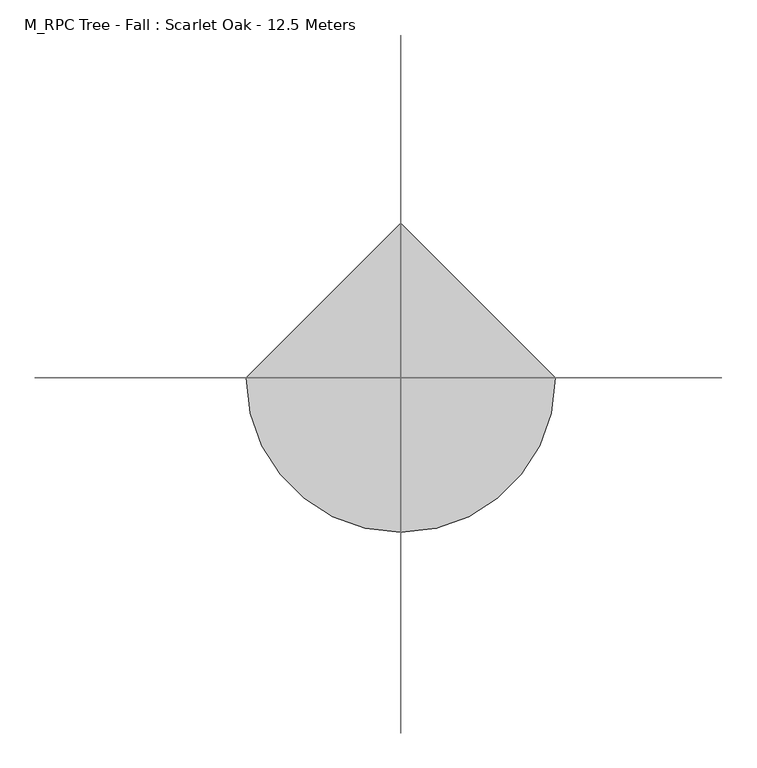
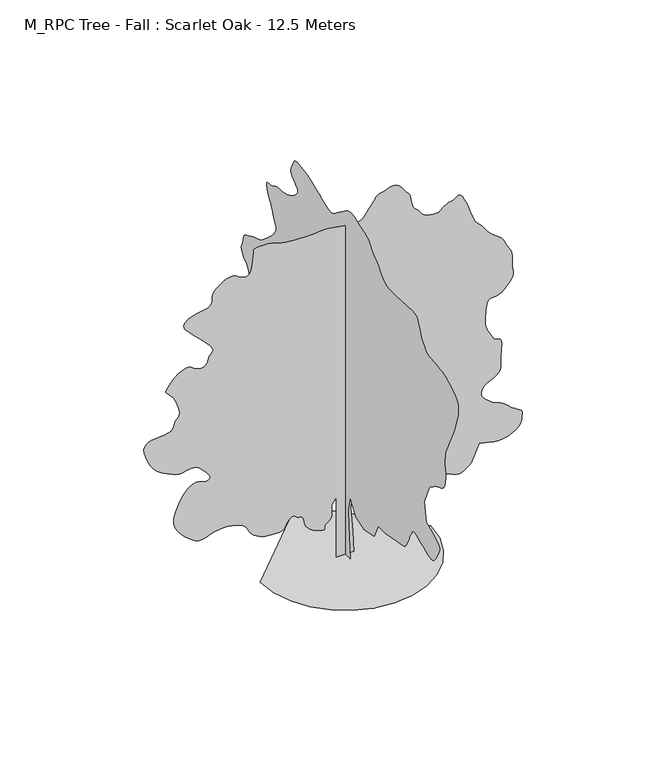
"""IFC4 building model written with IfcOpenShell, lengths in millimetres: geographic element geometry, M_RPC Tree - Fall : Scarlet Oak - 12.5 Meters."""

from ifc_helpers import new_model, si_unit, origin, place, context, project, spatial, triangles, source, transform, mapped, element, save


def m_rpc_tree_fall_scarlet_oak_12_5_meters_78a4568a(model_context):
    return source(origin(), model_context, "Body", "Tessellation", [
        triangles([(0.0172504, 306.0074844, 0.0), (0.0172504, -293.5650026, 0.0), (0.0172504, -196.8600042, 1141.1200275), (0.0172504, -177.5185068, 1682.6674953), (0.0172504, -293.5650026, 2185.5350567), (0.0172504, -603.0224945, 1682.6674953), (0.0172504, -1105.8875124, 1527.9400211), (0.0172504, -1686.1174301, 1663.3275421), (0.0172504, -1918.2099495, 2146.8525341), (0.0172504, -2324.3725124, 2146.8525341), (0.0172504, -3446.150116, 2359.6049549), (0.0172504, -3487.4249222, 2409.394939), (0.0172504, -3527.7000801, 2459.5225479), (0.0172504, -3565.9250725, 2510.3249702), (0.0172504, -3601.0999603, 2562.1500046), (0.0172504, -3632.2250954, 2615.3249565), (0.0172504, -3658.2749588, 2670.2000954), (0.0172504, -3678.2499023, 2727.0751122), (0.0172504, -3697.649881, 2785.6750237), (0.0172504, -3722.1251312, 2845.2748741), (0.0172504, -3750.8251236, 2905.7249634), (0.0172504, -3782.89991, 2966.8500114), (0.0172504, -3817.5251221, 3028.475029), (0.0172504, -3853.8249413, 3090.4500252), (0.0172504, -3890.9999977, 3152.5750122), (0.0172504, -3908.7000801, 3172.6499496), (0.0172504, -3933.1750397, 3188.8501236), (0.0172504, -3971.1750458, 3197.2499016), (0.0172504, -4029.4749756, 3193.9751015), (0.0172504, -4114.8499969, 3175.1500877), (0.0172504, -4234.0499886, 3136.8500999), (0.0172504, -4393.8501183, 3075.2250824), (0.0172504, -4562.5749939, 3002.6998581), (0.0172504, -4706.2499451, 2937.9750298), (0.0172504, -4828.2750549, 2886.4249786), (0.0172504, -4932.0251175, 2853.4999535), (0.0172504, -5020.8999252, 2844.5999153), (0.0172504, -5098.249855, 2865.125116), (0.0172504, -5167.5002792, 2920.4999336), (0.0172504, -5237.3750839, 3007.7251328), (0.0172504, -5309.5997452, 3113.9000473), (0.0172504, -5377.1002762, 3229.5499649), (0.0172504, -5432.7497864, 3345.1998825), (0.0172504, -5469.4498718, 3451.3750877), (0.0172504, -5480.1248016, 3538.6249947), (0.0172504, -5457.6250122, 3597.424894), (0.0172504, -5402.6498795, 3641.7000984), (0.0172504, -5323.3000717, 3691.0249947), (0.0172504, -5223.6747574, 3744.5999222), (0.0172504, -5107.774855, 3801.5499344), (0.0172504, -4979.7251129, 3861.0500816), (0.0172504, -4843.5499947, 3922.2251266), (0.0172504, -4703.3251236, 3984.2501198), (0.0172504, -4587.2749397, 4641.8500969), (0.0172504, -4877.3749649, 5318.7747665), (0.0172504, -4886.5249878, 5331.7001404), (0.0172504, -4900.7252838, 5347.4747589), (0.0172504, -4925.0999588, 5369.0251877), (0.0172504, -4964.6748688, 5399.20009), (0.0172504, -5024.5502838, 5440.8498734), (0.0172504, -5109.8247299, 5496.8999405), (0.0172504, -5225.5252258, 5570.225116), (0.0172504, -5351.0501221, 5636.6501312), (0.0172504, -5462.3497238, 5680.0498077), (0.0172504, -5559.4501923, 5715.3499786), (0.0172504, -5642.3497833, 5757.424736), (0.0172504, -5711.0252426, 5821.1499161), (0.0172504, -5765.4998245, 5921.4001923), (0.0172504, -5805.7502747, 6073.0752365), (0.0172504, -5829.0500153, 6222.0498642), (0.0172504, -5835.7501877, 6317.5748474), (0.0172504, -5830.6249191, 6379.6001312), (0.0172504, -5818.3750854, 6428.1000778), (0.0172504, -5803.7748138, 6483.0252136), (0.0172504, -5791.5499786, 6564.3249023), (0.0172504, -5786.4247101, 6692.0002487), (0.0172504, -5788.2251816, 6832.849791), (0.0172504, -5796.1252808, 6949.6752182), (0.0172504, -5813.8247818, 7056.3751007), (0.0172504, -5845.0502014, 7166.7747574), (0.0172504, -5893.550148, 7294.7750839), (0.0172504, -5963.0249771, 7454.2502335), (0.0172504, -6057.1750443, 7659.049942), (0.0172504, -6146.5748199, 7844.1752701), (0.0172504, -6206.1752518, 7955.8748474), (0.0172504, -6246.4751175, 8024.9502823), (0.0172504, -6277.9999374, 8082.1752777), (0.0172504, -6311.225235, 8158.3502792), (0.0172504, -6356.599791, 8284.2751511), (0.0172504, -6424.6752869, 8490.6997604), (0.0172504, -6498.0248795, 8729.4997192), (0.0172504, -6547.3747742, 8935.1499573), (0.0172504, -6565.2498459, 9112.3751862), (0.0172504, -6544.199968, 9265.925116), (0.0172504, -6476.8250107, 9400.5250397), (0.0172504, -6355.6498489, 9520.9002502), (0.0172504, -6173.2249374, 9631.8248749), (0.0172504, -5996.2252762, 9723.0001236), (0.0172504, -5879.7998245, 9785.7747803), (0.0172504, -5799.2250916, 9827.2001587), (0.0172504, -5729.8002594, 9854.4496582), (0.0172504, -5646.85009, 9874.575174), (0.0172504, -5525.6749283, 9894.699527), (0.0172504, -5341.575119, 9921.9501892), (0.0172504, -5144.0999634, 9943.4244598), (0.0172504, -4990.9500092, 9951.725116), (0.0172504, -4869.5998581, 9962.0244873), (0.0172504, -4767.5499825, 9989.5995483), (0.0172504, -4672.2499855, 10049.6505341), (0.0172504, -4571.2000488, 10157.425351), (0.0172504, -4451.8750648, 10328.0998169), (0.0172504, -4347.6750298, 10515.7499908), (0.0172504, -4286.1000092, 10666.5500885), (0.0172504, -4245.8501404, 10783.8254883), (0.0172504, -4205.5749825, 10871.0003998), (0.0172504, -4143.9999619, 10931.4501984), (0.0172504, -4039.7999268, 10968.5502594), (0.0172504, -3871.650016, 10985.7003754), (0.0172504, -2943.2749969, 10927.6748474), (0.0172504, -2772.1499771, 10930.6746643), (0.0172504, -2632.8250511, 10930.2746887), (0.0172504, -2514.4500092, 10937.3254211), (0.0172504, -2406.244986, 10962.6250397), (0.0172504, -2297.3600624, 11017.0496246), (0.0172504, -2176.9724979, 11111.3752625), (0.0172504, -2034.2550465, 11256.4745453), (0.0172504, -1896.7275398, 11403.0249023), (0.0172504, -1793.7050491, 11502.8746216), (0.0172504, -1717.0749882, 11568.5752625), (0.0172504, -1658.7125622, 11612.6248993), (0.0172504, -1610.5025688, 11647.5250946), (0.0172504, -1564.320068, 11685.7995026), (0.0172504, -1512.0500027, 11739.9996826), (0.0172504, -1461.8649845, 11804.0004272), (0.0172504, -1420.8125484, 11863.6002777), (0.0172504, -1379.087479, 11919.1503754), (0.0172504, -1326.8724976, 11970.9495392), (0.0172504, -1254.3574471, 12019.4000702), (0.0172504, -1151.7299904, 12064.7996246), (0.0172504, -1009.182514, 12107.4749268), (0.0172504, -849.1549999, 12154.4999634), (0.0172504, -699.9524792, 12206.6002716), (0.0172504, -560.5600064, 12254.6496643), (0.0172504, -429.9675053, 12289.4998627), (0.0172504, -307.1550161, 12302.0246796), (0.0172504, -191.1079934, 12283.0746735), (0.0172504, -80.8134993, 12223.5248199), (0.0172504, 499.4175176, 11798.0252106), (0.0172504, 562.2325061, 11740.8496307), (0.0172504, 623.0199657, 11688.7504852), (0.0172504, 689.217524, 11646.7751404), (0.0172504, 768.2749804, 11620.0500275), (0.0172504, 867.630035, 11613.6248383), (0.0172504, 994.7275097, 11632.5748444), (0.0172504, 1157.0125168, 11681.9753174), (0.0172504, 1341.1749676, 11755.3254913), (0.0172504, 1526.6899521, 11837.8251068), (0.0172504, 1710.1749733, 11922.0246185), (0.0172504, 1888.2475342, 12000.4500641), (0.0172504, 2057.5249924, 12065.6995697), (0.0172504, 2214.6200546, 12110.3003357), (0.0172504, 2356.1550201, 12126.8249084), (0.0172504, 2484.8875694, 12135.849939), (0.0172504, 2604.4750374, 12156.3754303), (0.0172504, 2712.9251038, 12178.575238), (0.0172504, 2808.1501053, 12192.6755402), (0.0172504, 2888.1748718, 12188.8501923), (0.0172504, 2950.9251114, 12157.2753754), (0.0172504, 2994.400074, 12088.1249451), (0.0172504, 3033.2500282, 12001.2500153), (0.0172504, 3077.8499222, 11921.1246735), (0.0172504, 3119.7499809, 11845.0502472), (0.0172504, 3150.5001389, 11770.3245758), (0.0172504, 3161.6000427, 11694.2745667), (0.0172504, 3144.6249161, 11614.1503876), (0.0172504, 3091.124984, 11527.2498779), (0.0172504, 3009.2500397, 11447.6245056), (0.0172504, 2921.5998665, 11385.2504059), (0.0172504, 2841.4251091, 11331.3502075), (0.0172504, 2781.8749649, 11277.1000305), (0.0172504, 2756.1750801, 11213.7248291), (0.0172504, 2777.4749428, 11132.4251404), (0.0172504, 2859.0249069, 11024.3747589), (0.0172504, 2971.6250107, 10916.7255157), (0.0172504, 3077.7999252, 10838.2000763), (0.0172504, 3178.2249001, 10782.3), (0.0172504, 3273.574894, 10742.6745117), (0.0172504, 3364.5248657, 10712.8251709), (0.0172504, 3451.7750633, 10686.4000397), (0.0172504, 3535.9498672, 10656.8995148), (0.0172504, 3620.024968, 10634.1753204), (0.0172504, 3706.4749237, 10626.6746155), (0.0172504, 3795.2750267, 10625.9502411), (0.0172504, 3886.4499847, 10623.5248077), (0.0172504, 3980.0000885, 10610.9499939), (0.0172504, 4075.9250473, 10579.7495728), (0.0172504, 4174.1998627, 10521.5252197), (0.0172504, 4275.775058, 10469.80047), (0.0172504, 4375.6250679, 10451.2504395), (0.0172504, 4465.0001358, 10446.8995422), (0.0172504, 4535.0999268, 10437.8245148), (0.0172504, 4577.0999794, 10405.075351), (0.0172504, 4582.2249573, 10329.6753021), (0.0172504, 4541.7001053, 10192.7255219), (0.0172504, 4481.7999825, 10048.5994354), (0.0172504, 4432.0751106, 9951.4995483), (0.0172504, 4388.424868, 9882.1247131), (0.0172504, 4346.8250816, 9821.224942), (0.0172504, 4303.1751297, 9749.5002502), (0.0172504, 4253.4249687, 9647.6750702), (0.0172504, 4193.550135, 9496.4499985), (0.0172504, 4130.2749275, 9347.6997757), (0.0172504, 4075.8250534, 9253.7502777), (0.0172504, 4034.1999779, 9195.999733), (0.0172504, 4009.500032, 9155.8498581), (0.0172504, 4005.7749687, 9114.7000443), (0.0172504, 4027.1001205, 9053.900267), (0.0172504, 4077.4999512, 8954.8999146), (0.0172504, 4167.2249977, 8823.6747849), (0.0172504, 4293.1248711, 8684.3501495), (0.0172504, 4439.3499573, 8545.349913), (0.0172504, 4589.9500671, 8415.1497208), (0.0172504, 4729.0750053, 8302.2002197), (0.0172504, 4840.7748734, 8214.9747299), (0.0172504, 4909.1747681, 8161.9000626), (0.0172504, 4969.9001312, 8128.6997635), (0.0172504, 5061.0747986, 8095.1500671), (0.0172504, 5170.5250946, 8060.9248306), (0.0172504, 5286.0750183, 8025.675238), (0.0172504, 5395.524733, 7989.0751465), (0.0172504, 5486.6999817, 7950.8001572), (0.0172504, 5547.4247635, 7910.4747116), (0.0172504, 5598.275148, 7876.9750122), (0.0172504, 5663.0252655, 7853.2997131), (0.0172504, 5734.1749924, 7830.2999542), (0.0172504, 5804.3247803, 7798.8251312), (0.0172504, 5866.0250839, 7749.7752182), (0.0172504, 5911.8001968, 7673.9751938), (0.0172504, 5934.2499893, 7562.325032), (0.0172504, 5952.6250305, 7450.1749008), (0.0172504, 5984.1998474, 7370.8500916), (0.0172504, 6018.4750809, 7312.1501862), (0.0172504, 6045.000206, 7261.899765), (0.0172504, 6053.2252853, 7207.9501511), (0.0172504, 6032.699794, 7138.074765), (0.0172504, 5972.9249542, 7040.1249298), (0.0172504, 5898.7248322, 6948.3747162), (0.0172504, 5838.7250061, 6893.5251572), (0.0172504, 5788.2001831, 6857.9500031), (0.0172504, 5742.4000717, 6824.0497467), (0.0172504, 5696.6249588, 6774.2498795), (0.0172504, 5646.1001358, 6690.9747299), (0.0172504, 5586.0997284, 6556.5997925), (0.0172504, 5520.7002319, 6421.9998688), (0.0172504, 5460.6998245, 6337.1498154), (0.0172504, 5411.5249191, 6283.075209), (0.0172504, 5378.6001846, 6240.824881), (0.0172504, 5367.3247101, 6191.4999847), (0.0172504, 5383.09991, 6116.0999359), (0.0172504, 5431.3748703, 5995.7247253), (0.0172504, 5495.5000259, 5864.0502045), (0.0172504, 5555.8748291, 5761.8250488), (0.0172504, 5613.5747955, 5680.5747757), (0.0172504, 5669.5498672, 5611.8249023), (0.0172504, 5724.8749786, 5547.1497803), (0.0172504, 5780.5250702, 5478.0749268), (0.0172504, 5837.5250793, 5396.1502762), (0.0172504, 5903.6751114, 5315.3499756), (0.0172504, 5980.6500641, 5249.4249298), (0.0172504, 6060.324852, 5189.6000931), (0.0172504, 6134.5999695, 5127.0498413), (0.0172504, 6195.3247513, 5053.0252899), (0.0172504, 6234.4002731, 4958.675235), (0.0172504, 6243.7002869, 4835.2499199), (0.0172504, 6251.5248093, 4738.3250221), (0.0172504, 6280.349794, 4706.349939), (0.0172504, 6313.2251129, 4704.825032), (0.0172504, 6333.2500534, 4699.2500816), (0.0172504, 6323.4750687, 4655.0998695), (0.0172504, 6267.0500244, 4537.8750481), (0.0172504, 6146.999794, 4313.0501083), (0.0172504, 6021.4748978, 4060.8750938), (0.0172504, 5945.6998718, 3875.3750793), (0.0172504, 5898.3248566, 3742.6250427), (0.0172504, 5858.0749878, 3648.7999557), (0.0172504, 5803.5998245, 3580.0000854), (0.0172504, 5713.6000854, 3522.3751144), (0.0172504, 5566.7747452, 3462.0500175), (0.0172504, 5397.250209, 3413.1000984), (0.0172504, 5248.0500137, 3392.5748978), (0.0172504, 5111.025238, 3390.9999939), (0.0172504, 4978.0752136, 3398.9000931), (0.0172504, 4841.0498566, 3406.7749031), (0.0172504, 4691.8499519, 3405.1999992), (0.0172504, 4522.3501236, 3384.6750893), (0.0172504, 4353.2999771, 3366.3000481), (0.0172504, 4207.2498802, 3370.2500977), (0.0172504, 4078.7998718, 3385.7000267), (0.0172504, 3962.5249924, 3401.8249146), (0.0172504, 3853.0249901, 3407.8001312), (0.0172504, 3744.8749054, 3392.799884), (0.0172504, 3632.6500694, 3346.0001244), (0.0172504, 3525.249939, 3296.2499634), (0.0172504, 3436.4251282, 3270.2000999), (0.0172504, 3368.249929, 3253.6249489), (0.0172504, 3322.75009, 3232.3250862), (0.0172504, 3301.9499062, 3192.0499283), (0.0172504, 3307.8751259, 3118.6500481), (0.0172504, 3342.5500443, 2997.8498634), (0.0172504, 3398.475119, 2869.5251381), (0.0172504, 3465.5750931, 2778.7248665), (0.0172504, 3542.0000793, 2719.2500084), (0.0172504, 3625.8499031, 2684.8000763), (0.0172504, 3715.274968, 2669.1248703), (0.0172504, 3808.4250961, 2665.9500641), (0.0172504, 3903.4251114, 2669.0498749), (0.0172504, 4270.9250633, 2262.8999565), (0.0172504, 4299.7250496, 2217.1674282), (0.0172504, 4327.3501076, 2170.5925095), (0.0172504, 4352.6250183, 2122.3249615), (0.0172504, 4374.3248566, 2071.5174522), (0.0172504, 4391.2999832, 2017.3300621), (0.0172504, 4402.3498901, 1958.9125523), (0.0172504, 4406.2999397, 1895.4200615), (0.0172504, 4405.6249809, 1829.2200325), (0.0172504, 4400.8999786, 1763.6974331), (0.0172504, 4388.0248924, 1699.5299835), (0.0172504, 4362.9999664, 1637.3900265), (0.0172504, 4321.7248695, 1577.9574623), (0.0172504, 4260.1501396, 1521.9075405), (0.0172504, 4174.1998627, 1469.9175453), (0.0172504, 4092.2249245, 1425.7650078), (0.0172504, 4034.5999535, 1391.4249527), (0.0172504, 3985.4250481, 1364.8675621), (0.0172504, 3928.800016, 1344.0599659), (0.0172504, 3848.8499542, 1326.9749622), (0.0172504, 3729.6499626, 1311.5799717), (0.0172504, 3555.3001396, 1295.8475018), (0.0172504, 3356.9750359, 1298.1024513), (0.0172504, 3174.2251442, 1332.8375404), (0.0172504, 3003.6500908, 1392.27243), (0.0172504, 2841.8750816, 1468.6199501), (0.0172504, 2685.525032, 1554.1049938), (0.0172504, 2531.1748604, 1640.9425713), (0.0172504, 2375.4949734, 1721.3500179), (0.0172504, 2236.6675461, 1794.4849434), (0.0172504, 2129.3050587, 1863.5599422), (0.0172504, 2044.6099377, 1926.8850014), (0.0172504, 1973.7875164, 1982.7650208), (0.0172504, 1908.0399307, 2029.5099873), (0.0172504, 1838.5700432, 2065.4300331), (0.0172504, 1756.5824604, 2088.8300583), (0.0172504, 1666.4174698, 2108.5650455), (0.0172504, 1577.6074837, 2133.0375343), (0.0172504, 1489.134977, 2159.8799366), (0.0172504, 1399.9875114, 2186.7200134), (0.0172504, 1309.1449459, 2211.1925022), (0.0172504, 1215.5975309, 2230.9274895), (0.0172504, 1118.3299942, 2243.5575325), (0.0172504, 1018.8625191, 2250.1549496), (0.0172504, 919.3925005, 2253.7074944), (0.0172504, 819.9250254, 2254.7225487), (0.0172504, 720.4574776, 2253.7074944), (0.0172504, 620.9900024, 2251.1700039), (0.0172504, 521.5199839, 2247.6174591), (0.0172504, 422.0525087, 2243.5575325), (0.0172504, 228.6430025, 1953.4425373), (0.0172504, 189.960498, 1508.6000679), (280.4450004, 0.0006008, 0.0092122), (-299.7850081, 0.0006008, 0.0092122), (-299.7850081, 0.0004756, 2127.5199932), (-454.5149895, 0.0004756, 1914.7700432), (-454.5149895, 0.0005007, 1682.6775238), (-450.9625174, 0.0005007, 1628.8274677), (-450.9625174, 0.0005007, 1575.1449886), (-458.0674979, 0.0005007, 1521.8024597), (-475.8274967, 0.0005257, 1468.967458), (-507.8000001, 0.0005257, 1416.8100311), (-557.5350094, 0.0005257, 1365.4949947), (-628.5824896, 0.0005257, 1315.1974834), (-684.2375227, 0.0005257, 1262.982502), (-699.6325132, 0.0005257, 1210.0900183), (-696.0799685, 0.0005257, 1162.9524885), (-694.8950117, 0.0005257, 1127.990015), (-717.3950191, 0.0005257, 1111.6375248), (-784.8900272, 0.0005257, 1120.3225325), (-918.6974848, 0.0005257, 1160.4700092), (-1071.3399845, 0.0005257, 1223.0050003), (-1185.4125275, 0.0005257, 1293.6575191), (-1267.3425556, 0.0005257, 1371.0799736), (-1323.5625252, 0.0005257, 1453.9125629), (-1360.49748, 0.0005007, 1540.8049335), (-1384.5749348, 0.0005007, 1630.4049877), (-1402.2250202, 0.0005007, 1721.3600464), (-1406.7350647, 0.0005007, 1746.1124599), (-1413.4449749, 0.0005007, 1770.19006), (-1424.5524364, 0.0005007, 1792.9174519), (-1442.2599312, 0.0005007, 1813.6099388), (-1468.7600578, 0.0005007, 1831.5975037), (-1506.2599491, 0.0005007, 1846.2025715), (-1556.9524944, 0.0005007, 1856.7475674), (-1607.6450397, 0.0005007, 1874.1124958), (-1647.5100483, 0.0005007, 1903.3224861), (-1682.3025467, 0.0004756, 1934.9000645), (-1717.7700039, 0.0004756, 1959.3725533), (-1759.6674465, 0.0004756, 1967.2675655), (-1813.7424889, 0.0004756, 1949.1099529), (-1885.7500122, 0.0005007, 1895.4274738), (-1949.0724552, 0.0005007, 1820.3199944), (-1984.9925011, 0.0005007, 1746.902528), (-2011.1000645, 0.0005007, 1679.2374722), (-2044.9875309, 0.0005007, 1621.382428), (-2104.2525181, 0.0005007, 1577.4025543), (-2206.4824699, 0.0005007, 1551.3499294), (-2369.2750042, 0.0005007, 1547.2900028), (-2549.149926, 0.0005007, 1559.2449417), (-2695.2000229, 0.0005007, 1578.979929), (-2813.8250496, 0.0005007, 1607.1750103), (-2911.4999016, 0.0005007, 1644.5025284), (-2994.6250603, 0.0005007, 1691.6425289), (-3069.600135, 0.0005007, 1749.2724415), (-3142.9250198, 0.0005007, 1818.0650448), (-3205.1000038, 0.0005007, 1893.5100037), (-3249.7248962, 0.0004756, 1969.2975288), (-3287.549913, 0.0004756, 2043.389954), (-3329.4499718, 0.0004756, 2113.7625481), (-3386.2249947, 0.0004756, 2178.3824409), (-3468.7249008, 0.0004756, 2235.2224308), (-3587.7499031, 0.0004756, 2282.2499382), (-3707.4248657, 0.0004756, 2317.9974655), (-3794.2500893, 0.0004506, 2343.2600224), (-3862.8249733, 0.0004506, 2359.3875263), (-3927.6750847, 0.0004506, 2367.7325111), (-4003.3251183, 0.0004506, 2369.6499813), (-4104.3750549, 0.0004506, 2366.4924706), (-4245.3498802, 0.0004506, 2359.6125126), (-4400.3500122, 0.0004506, 2335.1974331), (-4538.1250328, 0.0004756, 2289.8050003), (-4665.0501343, 0.0004756, 2240.3524956), (-4787.5749229, 0.0004756, 2203.7574909), (-4912.1501678, 0.0004756, 2196.9349422), (-5045.1501892, 0.0004756, 2236.7999508), (-5193.0498825, 0.0004506, 2340.2725594), (-5347.7997391, 0.0004506, 2478.6475433), (-5490.6747391, 0.0004506, 2615.9999153), (-5612.2498764, 0.0004256, 2758.4499413), (-5703.0251495, 0.0004256, 2912.049868), (-5753.5499725, 0.0004256, 3082.8999046), (-5754.3499237, 0.0004005, 3277.0999695), (-5695.9250015, 0.0004005, 3500.7249825), (-5598.1501556, 0.0003755, 3726.2748779), (-5489.1998291, 0.0003755, 3919.6999901), (-5372.1499969, 0.0003505, 4077.2499664), (-5250.0248932, 0.0003505, 4195.2000343), (-5125.8499146, 0.0003505, 4269.8501289), (-5002.6998734, 0.0003505, 4297.4998947), (-4883.6001663, 0.0003505, 4274.3751434), (-4771.2750458, 0.0003505, 4235.4749016), (-4671.8250114, 0.0003505, 4218.8750427), (-4593.3248611, 0.0003505, 4225.6499199), (-4543.9249695, 0.0003505, 4256.7750549), (-4531.7501312, 0.0003505, 4313.2750946), (-4564.9001427, 0.0003505, 4396.1749763), (-4651.5000893, 0.0003254, 4506.4749298), (-4752.500029, 0.0003254, 4617.0998634), (-4829.4749817, 0.0003254, 4702.3498924), (-4891.5502625, 0.0003254, 4765.2751213), (-4947.8747314, 0.0003254, 4808.9250732), (-5007.6001556, 0.0003254, 4836.325145), (-5079.8248169, 0.0003004, 4850.5498581), (-5173.7248993, 0.0003004, 4854.5999016), (-5270.0248352, 0.0003254, 4845.5248741), (-5349.7751999, 0.0003254, 4824.5999886), (-5422.3998367, 0.0003254, 4801.3249557), (-5497.39991, 0.0003254, 4785.1250725), (-5584.2248428, 0.0003254, 4785.5250481), (-5692.3752182, 0.0003254, 4811.9748871), (-5831.3248764, 0.0003004, 4873.9498833), (-5978.7751785, 0.0003004, 4948.0997177), (-6108.6248108, 0.0003004, 5012.4248611), (-6224.6252884, 0.0003004, 5078.4748993), (-6330.4502243, 0.0003004, 5157.6997147), (-6429.8749695, 0.0003004, 5261.5997681), (-6526.574881, 0.0002754, 5401.7249359), (-6624.2997299, 0.0002754, 5589.5750977), (-6705.1000305, 0.0002503, 5784.4998276), (-6749.7002151, 0.0002503, 5941.2001465), (-6759.8001801, 0.0002503, 6064.0752045), (-6737.074823, 0.0002253, 6157.4997345), (-6683.2252029, 0.0002253, 6225.9002106), (-6599.9500534, 0.0002253, 6273.6502029), (-6488.899855, 0.0002253, 6305.1750229), (-6357.7997177, 0.0002253, 6323.2750809), (-6219.2750336, 0.0002253, 6333.9500107), (-6082.4002487, 0.0002253, 6346.2748398), (-5956.3748016, 0.0002253, 6369.4501694), (-5850.3248795, 0.0002253, 6412.5998611), (-5773.3499268, 0.0002253, 6484.8251038), (-5734.5999664, 0.0002003, 6595.2997559), (-5705.9749695, 0.0002003, 6701.9752213), (-5661.749762, 0.0002003, 6771.4500504), (-5614.8497177, 0.0002003, 6825.7002274), (-5578.0752182, 0.0002003, 6886.6999924), (-5564.3248947, 0.0001752, 6976.4747452), (-5586.4252899, 0.0001752, 7116.9998886), (-5657.2500366, 0.0001752, 7330.2502441), (-5757.5497284, 0.0001502, 7540.3002136), (-5853.4752686, 0.0001502, 7672.5252823), (-5935.8498917, 0.0001502, 7750.975145), (-5995.5747345, 0.0001252, 7799.6250824), (-6023.4747757, 0.0001252, 7842.5247894), (-6010.4499893, 0.0001252, 7903.7251236), (-5947.3497711, 0.0001252, 8007.2002029), (-5845.6501648, 0.0001252, 8136.3248795), (-5728.0247864, 0.0001001, 8253.9502579), (-5602.2749039, 0.0001001, 8353.3000076), (-5476.1750427, 0.0001001, 8427.6251221), (-5357.5497253, 0.0001001, 8470.1248535), (-5254.1252243, 0.0001001, 8474.0751938), (-5173.7248993, 0.0001001, 8432.6998123), (-5094.9000595, 0.0001001, 8371.00009), (-4997.8001724, 0.0001001, 8322.8501221), (-4892.5751999, 0.0001001, 8294.6500992), (-4789.3751038, 0.0001001, 8292.850209), (-4698.375135, 0.0001001, 8323.8750595), (-4629.6999664, 0.0001001, 8394.1248413), (-4593.5001411, 0.0001001, 8510.0497421), (-4560.3251312, 0.0001001, 8620.5749725), (-4508.2251137, 7.51e-05, 8686.1000427), (-4458.4999512, 7.51e-05, 8730.3002518), (-4432.4500877, 7.51e-05, 8776.8747345), (-4451.4000938, 7.51e-05, 8849.4999527), (-4536.6501228, 7.51e-05, 8971.8750412), (-4709.5500343, 5.01e-05, 9167.6497192), (-4926.3498825, 5.01e-05, 9388.800174), (-5120.1502625, 2.5e-05, 9575.0998489), (-5277.4249649, 2.5e-05, 9731.9751572), (-5384.5998184, 2.5e-05, 9864.8246063), (-5428.2000641, 0.0, 9979.0746094), (-5394.6497864, 0.0, 10080.1254181), (-5270.4248108, 0.0, 10173.3755402), (-5104.7500397, 0.0, 10245.2246429), (-4956.3497955, 0.0, 10286.2744629), (-4825.8749107, 0.0, 10308.3754395), (-4714.0000534, -2.5e-05, 10323.3745239), (-4621.3998917, -2.5e-05, 10343.1000641), (-4548.7749641, -2.5e-05, 10379.4245911), (-4496.7749405, -2.5e-05, 10444.1497101), (-4470.8500694, -2.5e-05, 10520.7252686), (-4466.9000198, -2.5e-05, 10587.8246613), (-4471.4000359, -2.5e-05, 10650.1999237), (-4470.8500694, -2.5e-05, 10712.5751862), (-4451.6750771, -5.01e-05, 10779.6745789), (-4400.3500122, -5.01e-05, 10856.2501373), (-4303.3751175, -5.01e-05, 10947.0248291), (-4184.6750954, -5.01e-05, 11036.8495789), (-4076.1250351, -5.01e-05, 11106.7255463), (-3976.0500389, -7.51e-05, 11155.60047), (-3882.7249214, -7.51e-05, 11182.4999908), (-3794.4750755, -7.51e-05, 11186.3997528), (-3709.6000237, -7.51e-05, 11166.2498199), (-3626.4498665, -5.01e-05, 11121.1002502), (-3540.7248665, -5.01e-05, 11065.9001312), (-3452.3250298, -5.01e-05, 11022.8748505), (-3365.6000908, -5.01e-05, 11001.8249725), (-3284.9500717, -5.01e-05, 11012.5998962), (-3214.7999931, -5.01e-05, 11064.9746063), (-3159.5498772, -7.51e-05, 11168.7996643), (-3123.5750381, -7.51e-05, 11333.8500549), (-3102.0998955, -7.51e-05, 11511.0752838), (-3086.6999634, -0.0001001, 11648.0250641), (-3076.3750122, -0.0001001, 11749.4746857), (-3070.125103, -0.0001001, 11820.1250244), (-3066.9000092, -0.0001001, 11864.7246277), (-3065.7250809, -0.0001001, 11888.025531), (-3065.5500916, -0.0001001, 11894.7251221), (-3040.1248993, -0.0001001, 11898.674881), (-2971.0500458, -0.0001001, 11907.3755127), (-2869.1498703, -0.0001001, 11916.0505646), (-2745.2748734, -0.0001001, 11920.0003235), (-2610.2249771, -0.0001001, 11914.4750793), (-2474.8323692, -0.0001001, 11894.7251221), (-2349.935051, -0.0001001, 11856.0495758), (-2235.4100647, -0.0001001, 11813.0254578), (-2120.5474537, -0.0001001, 11781.8494537), (-2000.2725277, -0.0001001, 11760.1251984), (-1869.5075443, -0.0001001, 11745.5249268), (-1723.1824642, -0.0001001, 11735.675528), (-1556.2175102, -0.0001001, 11728.174823), (-1363.5400269, -0.0001001, 11720.6752808), (-1177.5749971, -0.0001001, 11719.599765), (-1024.4249702, -0.0001001, 11728.6747925), (-889.5449764, -0.0001001, 11741.475174), (-758.3875025, -0.0001001, 11751.5745575), (-616.4050352, -0.0001001, 11752.5244995), (-449.0450109, -0.0001001, 11737.9253906), (-241.763259, -0.0001001, 11701.3252991), (-32.2257492, -0.0001001, 11657.8000488), (136.7125037, -0.0001001, 11627.7995544), (271.8174929, -0.0001001, 11613.0248749), (379.8574825, -0.0001001, 11615.1503265), (467.5975121, -0.0001001, 11635.9246399), (541.8025031, -0.0001001, 11676.9744598), (609.2425, -0.0001001, 11739.9996826), (899.3575315, -0.0001252, 12107.4749268), (942.8899761, -0.0001252, 12164.1505371), (977.6249926, -0.0001252, 12217.4496094), (1008.9749685, -0.0001252, 12266.3245331), (1042.3575239, -0.0001252, 12309.7997864), (1083.1825029, -0.0001252, 12346.8498505), (1136.864982, -0.0001252, 12376.4503693), (1208.8150234, -0.0001252, 12397.6002411), (1297.0049892, -0.0001502, 12421.8499237), (1393.3149536, -0.0001502, 12454.2246918), (1494.0224693, -0.0001502, 12483.8752075), (1595.4100307, -0.0001502, 12499.9998047), (1693.7499584, -0.0001502, 12491.7747253), (1785.3225666, -0.0001502, 12448.349469), (1866.410059, -0.0001252, 12358.9246948), (1938.4149662, -0.0001252, 12256.9251068), (2004.3324543, -0.0001252, 12177.5752991), (2062.8075188, -0.0001252, 12112.7746033), (2112.4850098, -0.0001252, 12054.4246765), (2152.0125389, -0.0001252, 11994.3748535), (2180.0375725, -0.0001001, 11924.5000488), (2195.2049606, -0.0001001, 11836.6995941), (2205.7499565, -0.0001001, 11745.7004974), (2220.3550243, -0.0001001, 11669.9248901), (2238.3424438, -0.0001001, 11606.8252533), (2259.0349308, -7.51e-05, 11553.8749969), (2281.7599972, -7.51e-05, 11508.5254395), (2305.8374519, -7.51e-05, 11468.2755707), (2330.5924816, -7.51e-05, 11430.5499664), (2355.6274361, -7.51e-05, 11413.5754211), (2381.680061, -7.51e-05, 11394.2254395), (2409.760033, -7.51e-05, 11370.1501648), (2440.8876389, -7.51e-05, 11338.9753235), (2476.0724098, -7.51e-05, 11298.3254791), (2516.3248947, -7.51e-05, 11245.8251953), (2562.6749725, -7.51e-05, 11179.1246155), (2631.3751396, -5.01e-05, 11115.7249969), (2728.4750267, -5.01e-05, 11072.3253204), (2839.7749191, -5.01e-05, 11045.1246552), (2951.0751022, -5.01e-05, 11030.4755493), (3048.1749893, -5.01e-05, 11024.6003265), (3116.8748657, -5.01e-05, 11023.8247925), (3142.9250198, -5.01e-05, 11024.4003387), (3156.2750771, -5.01e-05, 11038.3250702), (3192.9998703, -5.01e-05, 11074.2252045), (3247.9750031, -5.01e-05, 11123.3501129), (3316.1499115, -7.51e-05, 11176.8503357), (3392.4249069, -7.51e-05, 11225.9752441), (3471.7750053, -7.51e-05, 11261.8997955), (3549.0749382, -7.51e-05, 11275.824527), (3618.3750687, -7.51e-05, 11292.800235), (3679.5501137, -7.51e-05, 11331.0746429), (3736.350135, -7.51e-05, 11371.7244873), (3792.4499084, -7.51e-05, 11395.8253418), (3851.6000771, -7.51e-05, 11384.3748779), (3917.5251228, -7.51e-05, 11318.4498322), (3993.9251106, -7.51e-05, 11179.1246155), (4065.8750793, -5.01e-05, 11015.4253052), (4119.5500008, -5.01e-05, 10883.1996552), (4160.3751251, -5.01e-05, 10773.6249481), (4193.7501228, -2.5e-05, 10677.9505554), (4225.0999535, -2.5e-05, 10587.3246918), (4259.8498672, -2.5e-05, 10493.0002167), (4303.3751175, -2.5e-05, 10386.1253448), (4348.1000038, 0.0, 10292.3496735), (4386.3749931, 0.0, 10232.749823), (4423.6500435, 0.0, 10191.7755798), (4465.325116, 0.0, 10153.8255707), (4516.799881, 0.0, 10103.3495819), (4583.4998795, 0.0, 10024.7997253), (4670.850071, 0.0, 9902.6002075), (4778.3749031, 2.5e-05, 9766.6003693), (4896.3999664, 2.5e-05, 9652.9247498), (5016.4501968, 2.5e-05, 9555.474884), (5130.075238, 5.01e-05, 9468.1999786), (5228.8000259, 5.01e-05, 9384.974826), (5304.2000748, 5.01e-05, 9299.6997986), (5347.7997391, 5.01e-05, 9206.3252655), (5382.0249756, 5.01e-05, 9114.7500412), (5429.774968, 7.51e-05, 9032.6498199), (5483.3001892, 7.51e-05, 8950.5501801), (5534.7749542, 7.51e-05, 8858.9749557), (5576.449736, 7.51e-05, 8748.4747238), (5600.5250107, 0.0001001, 8609.5250656), (5599.22509, 0.0001001, 8432.6998123), (5596.5752518, 0.0001001, 8262.7497208), (5611.174942, 0.0001252, 8138.7997284), (5627.1251312, 0.0001252, 8042.949765), (5628.5500443, 0.0001252, 7957.224765), (5599.5000732, 0.0001252, 7863.750238), (5524.1250229, 0.0001502, 7744.5249573), (5386.4752853, 0.0001502, 7581.6750137), (5223.124791, 0.0001502, 7444.9502197), (5081.4247192, 0.0001502, 7390.0750809), (4961.7000504, 0.0001502, 7378.1752258), (4864.3248894, 0.0001502, 7370.3501221), (4789.60009, 0.0001752, 7327.6498215), (4737.9000481, 0.0001752, 7211.2249512), (4709.5250359, 0.0001752, 6982.1249817), (4698.9251015, 0.0002003, 6728.5997589), (4700.5250038, 0.0002003, 6550.1751846), (4714.6000168, 0.0002253, 6424.9002731), (4741.5751144, 0.0002253, 6330.7252075), (4781.7249893, 0.0002253, 6245.7001648), (4835.3999107, 0.0002253, 6147.7997452), (4902.950148, 0.0002503, 6015.0752884), (4980.0250946, 0.0002503, 5899.6497757), (5057.7999985, 0.0002503, 5847.1500732), (5129.8002548, 0.0002503, 5825.7752151), (5189.6250916, 0.0002503, 5803.7248169), (5230.8499008, 0.0002503, 5749.200238), (5247.0250763, 0.0002754, 5630.3749329), (5231.7498459, 0.0002754, 5415.5002579), (5210.9999496, 0.0003004, 5178.6001831), (5207.8251434, 0.0003004, 5005.3247131), (5211.4499222, 0.0003004, 4881.0997375), (5210.9999496, 0.0003254, 4791.3999802), (5195.6497238, 0.0003254, 4721.6498772), (5154.5999039, 0.0003254, 4657.3000259), (5077.0249878, 0.0003254, 4583.8248596), (4983.2998947, 0.0003254, 4514.9249954), (4900.3997223, 0.0003254, 4468.3499313), (4827.3251129, 0.0003254, 4435.6498924), (4763.0499664, 0.0003505, 4408.3501053), (4706.5499268, 0.0003505, 4378.0249214), (4656.8250549, 0.0003505, 4336.1748596), (4612.8251244, 0.0003505, 4274.3751434), (4577.8749321, 0.0003505, 4202.8248596), (4558.1249748, 0.0003505, 4135.32491), (4557.0000435, 0.0003505, 4068.8498978), (4577.8749321, 0.0003755, 4000.3250107), (4624.1000175, 0.0003755, 3926.7501411), (4699.1000908, 0.0003755, 3845.024897), (4806.2499458, 0.0003755, 3752.1750412), (4919.8002823, 0.0003755, 3670.8000664), (5016.1252167, 0.0003755, 3617.5001221), (5101.6002319, 0.0004005, 3580.1250778), (5182.6999329, 0.0004005, 3546.4750969), (5265.8000931, 0.0004005, 3504.3500519), (5357.374736, 0.0004005, 3441.5751045), (5463.8252151, 0.0004005, 3346.0001244), (5576.8497116, 0.0004005, 3247.2750458), (5681.0497467, 0.0004005, 3176.6249977), (5772.3999847, 0.0004256, 3124.2249985), (5846.8250931, 0.0004256, 3080.3000633), (5900.2747375, 0.0004256, 3035.0249199), (5928.6997467, 0.0004256, 2978.5748772), (5928.0247879, 0.0004256, 2901.1499519), (5916.924884, 0.0004256, 2813.2500847), (5910.1997131, 0.0004506, 2730.7498878), (5898.0748718, 0.0004506, 2651.975045), (5870.7247971, 0.0004506, 2575.2500771), (5818.350087, 0.0004506, 2498.8349739), (5731.1251785, 0.0004506, 2421.0750401), (5599.22509, 0.0004506, 2340.2725594), (5441.7248199, 0.0004756, 2274.8624531), (5284.2501297, 0.0004756, 2240.917432), (5126.7498596, 0.0004756, 2233.1924675), (4969.2501709, 0.0004756, 2246.4425308), (4811.7748993, 0.0004756, 2275.4250641), (4654.2749199, 0.0004756, 2314.8975094), (4496.7749405, 0.0004506, 2359.6125126), (4225.9998985, 0.0005007, 1760.042569), (4159.6498787, 0.0005007, 1702.5250042), (4092.9248817, 0.0005007, 1648.0549278), (4025.5499245, 0.0005007, 1599.675032), (3957.1500298, 0.0005007, 1560.4274277), (3887.3999268, 0.0005007, 1533.3625099), (3815.9499275, 0.0005007, 1521.5225349), (3742.4750519, 0.0005007, 1527.9500496), (3682.5999275, 0.0005007, 1542.5525013), (3644.6999153, 0.0005007, 1554.7899811), (3617.6501129, 0.0005007, 1567.0274609), (3590.2500412, 0.0005007, 1581.6300579), (3551.3250916, 0.0005007, 1600.9724819), (3489.750071, 0.0005007, 1627.4175247), (3394.3500801, 0.0005007, 1663.3375706), (3270.0751076, 0.0005007, 1715.4949974), (3134.2999649, 0.0005007, 1784.5699963), (2994.450071, 0.0005007, 1863.794957), (2857.9999695, 0.0004756, 1946.40256), (2732.3500809, 0.0004756, 2025.6275208), (2624.9999474, 0.0004756, 2094.7025196), (2543.3499893, 0.0004756, 2146.8625626), (2474.2126396, 0.0004756, 2192.817461), (2400.0074306, 0.0004756, 2246.8925034), (2321.5700672, 0.0004756, 2307.7374813), (2239.7525322, 0.0004506, 2373.9924488), (2155.3950359, 0.0004506, 2444.3074883), (2069.3475266, 0.0004506, 2517.3251244), (1982.4550106, 0.0004506, 2591.6999451), (1963.1124413, 0.0004256, 2881.8249687), (1576.2924477, 0.0004256, 2920.4999336), (880.0150349, 0.0004256, 2862.474987), (415.8325032, 0.0004506, 2611.0499268), (222.4215072, 0.0004756, 2146.8625626), (183.7397477, 0.0005007, 1605.3124786), (241.7622416, 0.0005507, 715.6274672), (-2855.9000977, 0.0, 0.0224297), (-2780.4000549, -654.3849844, 0.0224297), (-2565.3750984, -1255.3350037, 0.0224297), (-2228.0500488, -1785.6274899, 0.0224297), (-1785.6274899, -2228.0500488, 0.0224297), (-1255.3350037, -2565.3750984, 0.0224297), (-654.3849844, -2780.4000549, 0.0224297), (0.0001248, -2855.9000977, 0.0224297), (654.3849844, -2780.4000549, 0.0224297), (1255.3350037, -2565.3750984, 0.0224297), (1785.6274899, -2228.0500488, 0.0224297), (2228.0500488, -1785.6274899, 0.0224297), (2565.3750984, -1255.3350037, 0.0224297), (2780.4000549, -654.3849844, 0.0224297), (2855.9000977, 0.0002503, 0.0224297), (-0.0003745, 2855.9000977, 0.0224297)], [[1, 2, 3], [368, 1, 3], [368, 3, 4], [367, 368, 4], [367, 4, 5], [277, 278, 279], [366, 367, 5], [276, 277, 279], [276, 279, 280], [7, 8, 9], [6, 7, 9], [5, 6, 9], [315, 316, 317], [201, 202, 203], [200, 201, 203], [200, 203, 204], [199, 200, 204], [199, 204, 205], [198, 199, 205], [198, 205, 206], [198, 206, 207], [197, 198, 207], [197, 207, 208], [275, 276, 280], [196, 197, 208], [195, 196, 208], [194, 195, 208], [194, 208, 209], [193, 194, 209], [192, 193, 209], [192, 209, 210], [191, 192, 210], [191, 210, 211], [191, 211, 212], [190, 191, 212], [190, 212, 213], [190, 213, 214], [189, 190, 214], [189, 214, 215], [188, 189, 215], [187, 188, 215], [186, 187, 215], [10, 11, 12], [314, 315, 317], [10, 12, 13], [10, 13, 14], [10, 14, 15], [10, 15, 16], [10, 16, 17], [10, 17, 18], [10, 18, 19], [10, 19, 20], [10, 20, 21], [10, 21, 22], [185, 186, 215], [185, 215, 216], [275, 280, 281], [10, 22, 23], [167, 168, 169], [166, 167, 169], [165, 166, 169], [165, 169, 170], [164, 165, 170], [164, 170, 171], [163, 164, 171], [163, 171, 172], [163, 172, 173], [163, 173, 174], [163, 174, 175], [163, 175, 176], [163, 176, 177], [163, 177, 178], [163, 178, 179], [163, 179, 180], [162, 163, 180], [161, 162, 180], [160, 161, 180], [159, 160, 180], [159, 180, 181], [158, 159, 181], [157, 158, 181], [156, 157, 181], [156, 181, 182], [155, 156, 182], [154, 155, 182], [154, 182, 183], [9, 10, 23], [9, 23, 24], [9, 24, 25], [45, 46, 47], [44, 45, 47], [44, 47, 48], [43, 44, 48], [43, 48, 49], [42, 43, 49], [42, 49, 50], [41, 42, 50], [40, 41, 50], [40, 50, 51], [39, 40, 51], [38, 39, 51], [37, 38, 51], [36, 37, 51], [35, 36, 51], [34, 35, 51], [33, 34, 51], [33, 51, 52], [32, 33, 52], [32, 52, 53], [31, 32, 53], [30, 31, 53], [29, 30, 53], [28, 29, 53], [28, 53, 54], [27, 28, 54], [26, 27, 54], [5, 9, 25], [5, 25, 26], [5, 26, 54], [5, 54, 55], [366, 5, 55], [365, 366, 55], [364, 365, 55], [363, 364, 55], [362, 363, 55], [361, 362, 55], [361, 55, 56], [153, 154, 183], [153, 183, 184], [313, 314, 317], [360, 361, 56], [184, 185, 216], [153, 184, 216], [152, 153, 216], [152, 216, 217], [243, 244, 245], [242, 243, 245], [242, 245, 246], [241, 242, 246], [241, 246, 247], [241, 247, 248], [240, 241, 248], [240, 248, 249], [240, 249, 250], [239, 240, 250], [239, 250, 251], [238, 239, 251], [237, 238, 251], [236, 237, 251], [235, 236, 251], [234, 235, 251], [233, 234, 251], [232, 233, 251], [231, 232, 251], [230, 231, 251], [229, 230, 251], [228, 229, 251], [228, 251, 252], [227, 228, 252], [226, 227, 252], [226, 252, 253], [226, 253, 254], [226, 254, 255], [226, 255, 256], [226, 256, 257], [225, 226, 257], [224, 225, 257], [223, 224, 257], [222, 223, 257], [222, 257, 258], [221, 222, 258], [220, 221, 258], [115, 116, 117], [114, 115, 117], [114, 117, 118], [113, 114, 118], [113, 118, 119], [112, 113, 119], [111, 112, 119], [110, 111, 119], [152, 217, 218], [313, 317, 318], [313, 318, 319], [313, 319, 320], [313, 320, 321], [313, 321, 322], [313, 322, 323], [313, 323, 324], [313, 324, 325], [313, 325, 326], [313, 326, 327], [313, 327, 328], [313, 328, 329], [313, 329, 330], [313, 330, 331], [313, 331, 332], [313, 332, 333], [313, 333, 334], [313, 334, 335], [313, 335, 336], [313, 336, 337], [313, 337, 338], [313, 338, 339], [313, 339, 340], [313, 340, 341], [312, 313, 341], [312, 341, 342], [312, 342, 343], [311, 312, 343], [311, 343, 344], [311, 344, 345], [310, 311, 345], [310, 345, 346], [310, 346, 347], [310, 347, 348], [309, 310, 348], [309, 348, 349], [309, 349, 350], [308, 309, 350], [308, 350, 351], [307, 308, 351], [307, 351, 352], [307, 352, 353], [307, 353, 354], [307, 354, 355], [307, 355, 356], [307, 356, 357], [307, 357, 358], [306, 307, 358], [306, 358, 359], [306, 359, 360], [306, 360, 56], [305, 306, 56], [305, 56, 57], [304, 305, 57], [303, 304, 57], [302, 303, 57], [301, 302, 57], [301, 57, 58], [301, 58, 59], [110, 119, 120], [109, 110, 120], [109, 120, 121], [301, 59, 60], [300, 301, 60], [300, 60, 61], [151, 152, 218], [109, 121, 122], [300, 61, 62], [145, 146, 147], [144, 145, 147], [143, 144, 147], [143, 147, 148], [142, 143, 148], [141, 142, 148], [140, 141, 148], [140, 148, 149], [139, 140, 149], [138, 139, 149], [137, 138, 149], [136, 137, 149], [135, 136, 149], [134, 135, 149], [133, 134, 149], [132, 133, 149], [132, 149, 150], [131, 132, 150], [130, 131, 150], [129, 130, 150], [128, 129, 150], [127, 128, 150], [126, 127, 150], [126, 150, 151], [126, 151, 218], [125, 126, 218], [124, 125, 218], [123, 124, 218], [123, 218, 219], [122, 123, 219], [109, 122, 219], [108, 109, 219], [108, 219, 220], [108, 220, 258], [108, 258, 259], [108, 259, 260], [108, 260, 261], [108, 261, 262], [107, 108, 262], [107, 262, 263], [107, 263, 264], [106, 107, 264], [106, 264, 265], [106, 265, 266], [106, 266, 267], [106, 267, 268], [105, 106, 268], [104, 105, 268], [103, 104, 268], [102, 103, 268], [101, 102, 268], [100, 101, 268], [99, 100, 268], [98, 99, 268], [97, 98, 268], [96, 97, 268], [95, 96, 268], [94, 95, 268], [93, 94, 268], [92, 93, 268], [91, 92, 268], [90, 91, 268], [89, 90, 268], [88, 89, 268], [87, 88, 268], [86, 87, 268], [85, 86, 268], [84, 85, 268], [83, 84, 268], [82, 83, 268], [81, 82, 268], [80, 81, 268], [79, 80, 268], [78, 79, 268], [77, 78, 268], [76, 77, 268], [75, 76, 268], [74, 75, 268], [73, 74, 268], [72, 73, 268], [71, 72, 268], [70, 71, 268], [69, 70, 268], [68, 69, 268], [67, 68, 268], [66, 67, 268], [65, 66, 268], [64, 65, 268], [63, 64, 268], [62, 63, 268], [300, 62, 268], [299, 300, 268], [298, 299, 268], [297, 298, 268], [296, 297, 268], [295, 296, 268], [294, 295, 268], [293, 294, 268], [292, 293, 268], [291, 292, 268], [290, 291, 268], [289, 290, 268], [288, 289, 268], [287, 288, 268], [286, 287, 268], [285, 286, 268], [284, 285, 268], [283, 284, 268], [282, 283, 268], [281, 282, 268], [275, 281, 268], [275, 268, 269], [274, 275, 269], [274, 269, 270], [274, 270, 271], [273, 274, 271], [272, 273, 271], [802, 369, 370], [802, 370, 371], [801, 802, 371], [800, 801, 371], [575, 576, 577], [799, 800, 371], [574, 575, 577], [383, 384, 385], [383, 385, 386], [382, 383, 386], [382, 386, 387], [381, 382, 387], [381, 387, 388], [794, 795, 796], [510, 511, 512], [574, 577, 578], [573, 574, 578], [572, 573, 578], [572, 578, 579], [571, 572, 579], [571, 579, 580], [570, 571, 580], [570, 580, 581], [570, 581, 582], [569, 570, 582], [569, 582, 583], [569, 583, 584], [568, 569, 584], [568, 584, 585], [509, 510, 512], [509, 512, 513], [508, 509, 513], [508, 513, 514], [508, 514, 515], [507, 508, 515], [507, 515, 516], [507, 516, 517], [507, 517, 518], [507, 518, 519], [507, 519, 520], [507, 520, 521], [507, 521, 522], [506, 507, 522], [506, 522, 523], [505, 506, 523], [505, 523, 524], [504, 505, 524], [568, 585, 586], [504, 524, 525], [538, 539, 540], [538, 540, 541], [537, 538, 541], [537, 541, 542], [536, 537, 542], [536, 542, 543], [536, 543, 544], [535, 536, 544], [535, 544, 545], [535, 545, 546], [534, 535, 546], [534, 546, 547], [533, 534, 547], [533, 547, 548], [381, 388, 389], [380, 381, 389], [380, 389, 390], [380, 390, 391], [380, 391, 392], [380, 392, 393], [379, 380, 393], [378, 379, 393], [377, 378, 393], [376, 377, 393], [375, 376, 393], [374, 375, 393], [373, 374, 393], [372, 373, 393], [372, 393, 394], [372, 394, 395], [372, 395, 396], [372, 396, 397], [372, 397, 398], [371, 372, 398], [371, 398, 399], [532, 533, 548], [371, 399, 400], [567, 568, 586], [567, 586, 587], [657, 658, 659], [657, 659, 660], [656, 657, 660], [656, 660, 661], [655, 656, 661], [655, 661, 662], [654, 655, 662], [654, 662, 663], [653, 654, 663], [652, 653, 663], [651, 652, 663], [650, 651, 663], [649, 650, 663], [649, 663, 664], [648, 649, 664], [647, 648, 664], [647, 664, 665], [647, 665, 666], [647, 666, 667], [647, 667, 668], [647, 668, 669], [793, 794, 796], [713, 714, 715], [713, 715, 716], [712, 713, 716], [712, 716, 717], [711, 712, 717], [646, 647, 669], [711, 717, 718], [567, 587, 588], [645, 646, 669], [645, 669, 670], [750, 751, 752], [749, 750, 752], [748, 749, 752], [748, 752, 753], [747, 748, 753], [747, 753, 754], [747, 754, 755], [747, 755, 756], [747, 756, 757], [747, 757, 758], [747, 758, 759], [747, 759, 760], [746, 747, 760], [746, 760, 761], [746, 761, 762], [745, 746, 762], [745, 762, 763], [745, 763, 764], [744, 745, 764], [743, 744, 764], [743, 764, 765], [742, 743, 765], [741, 742, 765], [741, 765, 766], [740, 741, 766], [739, 740, 766], [738, 739, 766], [737, 738, 766], [736, 737, 766], [735, 736, 766], [644, 645, 670], [567, 588, 589], [792, 793, 796], [371, 400, 401], [371, 401, 402], [371, 402, 403], [371, 403, 404], [371, 404, 405], [799, 371, 405], [799, 405, 406], [766, 767, 768], [488, 489, 490], [488, 490, 491], [487, 488, 491], [487, 491, 492], [486, 487, 492], [486, 492, 493], [485, 486, 493], [485, 493, 494], [485, 494, 495], [484, 485, 495], [483, 484, 495], [483, 495, 496], [482, 483, 496], [481, 482, 496], [480, 481, 496], [479, 480, 496], [479, 496, 497], [478, 479, 497], [477, 478, 497], [476, 477, 497], [475, 476, 497], [474, 475, 497], [473, 474, 497], [472, 473, 497], [471, 472, 497], [471, 497, 498], [470, 471, 498], [469, 470, 498], [469, 498, 499], [468, 469, 499], [468, 499, 500], [468, 500, 501], [468, 501, 502], [468, 502, 503], [467, 468, 503], [466, 467, 503], [466, 503, 504], [466, 504, 525], [465, 466, 525], [465, 525, 526], [464, 465, 526], [463, 464, 526], [735, 766, 768], [735, 768, 769], [735, 769, 770], [735, 770, 771], [735, 771, 772], [735, 772, 773], [735, 773, 774], [735, 774, 775], [735, 775, 776], [735, 776, 777], [735, 777, 778], [735, 778, 779], [735, 779, 780], [735, 780, 781], [735, 781, 782], [735, 782, 783], [735, 783, 784], [735, 784, 785], [735, 785, 786], [735, 786, 787], [735, 787, 788], [735, 788, 789], [735, 789, 790], [735, 790, 791], [735, 791, 792], [735, 792, 796], [734, 735, 796], [733, 734, 796], [732, 733, 796], [731, 732, 796], [731, 796, 797], [730, 731, 797], [567, 589, 590], [455, 456, 457], [454, 455, 457], [453, 454, 457], [453, 457, 458], [452, 453, 458], [451, 452, 458], [451, 458, 459], [450, 451, 459], [449, 450, 459], [448, 449, 459], [447, 448, 459], [446, 447, 459], [445, 446, 459], [444, 445, 459], [443, 444, 459], [442, 443, 459], [441, 442, 459], [440, 441, 459], [439, 440, 459], [438, 439, 459], [437, 438, 459], [437, 459, 460], [436, 437, 460], [435, 436, 460], [434, 435, 460], [434, 460, 461], [433, 434, 461], [432, 433, 461], [431, 432, 461], [430, 431, 461], [429, 430, 461], [428, 429, 461], [428, 461, 462], [427, 428, 462], [411, 412, 413], [411, 413, 414], [410, 411, 414], [410, 414, 415], [409, 410, 415], [409, 415, 416], [409, 416, 417], [408, 409, 417], [408, 417, 418], [408, 418, 419], [408, 419, 420], [408, 420, 421], [408, 421, 422], [408, 422, 423], [408, 423, 424], [408, 424, 425], [408, 425, 426], [407, 408, 426], [407, 426, 427], [407, 427, 462], [406, 407, 462], [799, 406, 462], [799, 462, 463], [799, 463, 526], [798, 799, 526], [798, 526, 527], [798, 527, 528], [798, 528, 529], [798, 529, 530], [798, 530, 531], [797, 798, 531], [730, 797, 531], [729, 730, 531], [728, 729, 531], [728, 531, 532], [728, 532, 548], [728, 548, 549], [728, 549, 550], [727, 728, 550], [726, 727, 550], [725, 726, 550], [724, 725, 550], [723, 724, 550], [722, 723, 550], [721, 722, 550], [720, 721, 550], [719, 720, 550], [718, 719, 550], [711, 718, 550], [710, 711, 550], [709, 710, 550], [708, 709, 550], [707, 708, 550], [706, 707, 550], [705, 706, 550], [704, 705, 550], [703, 704, 550], [702, 703, 550], [701, 702, 550], [701, 550, 551], [701, 551, 552], [701, 552, 553], [701, 553, 554], [701, 554, 555], [701, 555, 556], [701, 556, 557], [701, 557, 558], [701, 558, 559], [700, 701, 559], [699, 700, 559], [698, 699, 559], [697, 698, 559], [696, 697, 559], [617, 618, 619], [616, 617, 619], [615, 616, 619], [615, 619, 620], [614, 615, 620], [613, 614, 620], [613, 620, 621], [612, 613, 621], [612, 621, 622], [611, 612, 622], [610, 611, 622], [609, 610, 622], [608, 609, 622], [607, 608, 622], [606, 607, 622], [605, 606, 622], [604, 605, 622], [604, 622, 623], [604, 623, 624], [604, 624, 625], [604, 625, 626], [604, 626, 627], [604, 627, 628], [604, 628, 629], [604, 629, 630], [604, 630, 631], [604, 631, 632], [603, 604, 632], [603, 632, 633], [602, 603, 633], [602, 633, 634], [602, 634, 635], [602, 635, 636], [602, 636, 637], [602, 637, 638], [602, 638, 639], [602, 639, 640], [602, 640, 641], [601, 602, 641], [643, 644, 670], [643, 670, 671], [567, 590, 591], [566, 567, 591], [692, 693, 694], [692, 694, 695], [691, 692, 695], [691, 695, 696], [690, 691, 696], [680, 681, 682], [689, 690, 696], [679, 680, 682], [679, 682, 683], [678, 679, 683], [559, 560, 561], [559, 561, 562], [559, 562, 563], [566, 591, 592], [642, 643, 671], [642, 671, 672], [642, 672, 673], [642, 673, 674], [642, 674, 675], [642, 675, 676], [600, 601, 641], [688, 689, 696], [687, 688, 696], [686, 687, 696], [685, 686, 696], [684, 685, 696], [683, 684, 696], [678, 683, 696], [677, 678, 696], [676, 677, 696], [642, 676, 696], [641, 642, 696], [600, 641, 696], [599, 600, 696], [598, 599, 696], [597, 598, 696], [596, 597, 696], [595, 596, 696], [594, 595, 696], [593, 594, 696], [592, 593, 696], [566, 592, 696], [565, 566, 696], [564, 565, 696], [564, 696, 559], [564, 559, 563], [817, 818, 803], [816, 817, 803], [816, 803, 804], [815, 816, 804], [815, 804, 805], [815, 805, 806], [814, 815, 806], [813, 814, 806], [813, 806, 807], [813, 807, 808], [813, 808, 809], [813, 809, 810], [813, 810, 811], [813, 811, 812]], closed=False),
    ])


if __name__ == "__main__":
    model = new_model("IFC4")
    model_context = context("Model", 3, world=origin())
    ifc_project = project(units=[si_unit("LENGTHUNIT", "METRE", prefix="MILLI")], contexts=[model_context])
    site = spatial("IfcSite", under=ifc_project)
    building = spatial("IfcBuilding", under=site)
    placement = place(None, origin())
    m_rpc_tree_fall_scarlet_oak_12_5_meters_shape = m_rpc_tree_fall_scarlet_oak_12_5_meters_78a4568a(model_context)
    element("IfcGeographicElement", 1, ObjectType="M_RPC Tree - Fall : Scarlet Oak - 12.5 Meters", at=placement, inside=building, context=model_context, shape_type="MappedRepresentation", body=[
        mapped(m_rpc_tree_fall_scarlet_oak_12_5_meters_shape, transform((0.0, 0.0, 0.0), x_axis=(1.0, 0.0, 0.0), y_axis=(0.0, 1.0, 0.0), z_axis=(0.0, 0.0, 1.0))),
    ])
    save(model, "model.ifc")

# Revit data of these elements
# Type "M_RPC Tree - Fall : Scarlet Oak - 12.5 Meters"
#   built-in parameter 1005198 = "{2, 15},{39, RPC-16-FXGN-QL00-PPP3-E000-ST1L-LVER-AU},{1, 0},{1, 0},{2, 13},{1, 8},{5, Color},{1, 0},{1, 0},{3, 0.8},{3, 0.8},{3, 0.8},{1, 8},{7, BBoxMin},{1, 0},{1, 0},{1, 0},{1, 0},{1, 0},{1, 8},{7, BBoxMax},{1, 0},{1, 0},{1, 0},{1, 0},{1, 0},{2, 11},{9, RPCTypeId},{1, 0},{1, 0},{39, RPC-16-FXGN-QL00-PPP3-E000-ST1L-LVER-AU},{1, 6},{14, RPCPlantHeight},{1, 0},{1, 0},{7, 41.0105},{2, 11},{7, keyword},{1, 0},{1, 0},{39, :RPCs:Fall Trees [General]:Geometry:RPC},{2, 11},{8, category},{1, 0},{1, 0},{20, Fall Trees [General]},{2, 11},{12, LocalizedUID},{1, 0},{1, 0},{18, Scarlet Oak [Fall]},{2, 14},{6, Height},{1, 0},{1, 0},{7, 41.0105},{1, 2},{16, Cast Reflections},{1, 0},{1, 0},{1, 0},{1, 2},{12, Cast Shadows},{1, 0},{1, 0},{1, 1},{1, 2},{9, Lock View},{1, 0},{1, 0},{1, 0},{1, 4},{5, ViewC},{1, 0},{1, 0},{1, 0},{21, assetlibrary_base.fbx},{1, 5},"
#   built-in parameter 1005195 = "RPC-16-FXGN-QL00-PPP3-E000-ST1L-LVER-AU"
#   Type Comments = "Scarlet Oak"
#   Height = 41.010499 ft
#   Default Elevation = 0
